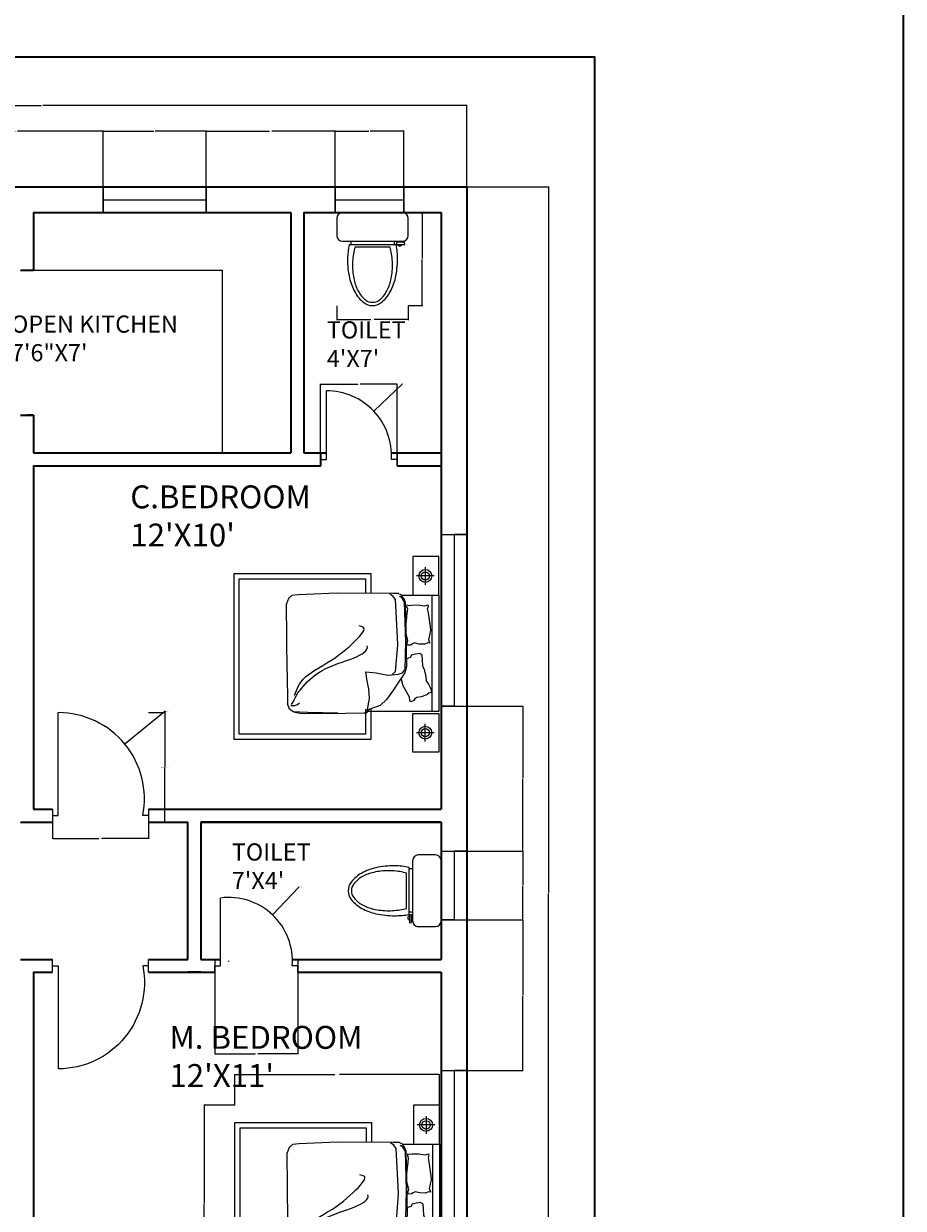
# Model space of a CAD drawing. Units: inches. Extents: x 1976 to 2558, y -977 to 2909.
# Tile 6 of 8: x 2251 to 2558, y 2026 to 2441. Entities that reach past the tile are written whole.
import ezdxf

# ---------------------------------------------------------------- set-up
doc = ezdxf.new("R2010")
doc.units = ezdxf.units.IN
for name, color, linetype, lineweight in [('A-ANNO-DIMS', 2, 'Continuous', 18), ('A-ANNO-TTLB', 7, 'Continuous', 35), ('A-AREA-IDEN', 7, 'Continuous', 18), ('A-DOOR', 3, 'Continuous', 18), ('A-FLOR-FIXT', 9, 'Continuous', 18), ('A-FURN', 8, 'Continuous', 13), ('A-GLAZ', 4, 'Continuous', 18), ('A-WALL', 7, 'Continuous', 35)]:
    doc.layers.add(name, color=color, linetype=linetype, lineweight=lineweight)
doc.styles.get("Standard").update_dxf_attribs({"font": 'arial.ttf'})
doc.dimstyles.get("Standard").update_dxf_attribs({"dimtxt": 0.18, "dimasz": 0.18, "dimexe": 0.18, "dimexo": 0.0625, "dimgap": 0.09, "dimtad": 0, "dimtih": 1, "dimtoh": 1, "dimdec": 4, "dimzin": 0, "dimdsep": 46, "dimtxsty": 'Standard', "dimcen": 0.09, "dimadec": 0, "dimazin": 0, "dimtfac": 1, "dimtdec": 4, "dimtofl": 0, "dimtmove": 0, "dimatfit": 3, "dimfxl": 1, "dimtolj": 1, "dimtzin": 0, "dimarcsym": 0})

# ---------------------------------------------------------------- blocks, each defined once
blk = doc.blocks.new('A$C238700B9')
for p, q in [((0, 0.61), (0, 0.49)), ((0.25, 0.65), (0.04, 0.65)), ((0.46, 0.65), (0.25, 0.65)), ((0.5, 0.49), (0.5, 0.61)), ((0.04, 0.45), (0.46, 0.45)), ((0.4166, 0.4252), (0.0876, 0.4252)), ((0.0974, 0.45), (0.0974, 0.4252)), ((0.401, 0.45), (0.401, 0.4252)), ((0.473, 0.4434), (0.419, 0.4434)), ((0.419, 0.4434), (0.419, 0.428)), ((0.419, 0.428), (0.4756, 0.428)), ((0.4337, 0.4434), (0.4337, 0.45)), ((0.446, 0.45), (0.446, 0.4434)), ((0.4756, 0.428), (0.473, 0.4434)), ((0.3733, 0.4074), (0.1267, 0.4074))]:
    blk.add_line(p, q)
for centre, radius, start, end in [((0.04, 0.61), 0.04, 90, 180), ((0.46, 0.61), 0.04, 0, 90), ((0.04, 0.49), 0.04, 180, 270), ((0.6767, 0.3001), 0.6022, 168.01944, 177.63471), ((-0.1767, 0.325), 0.6017, 0, 9.58156), ((0.4403, 0.434), 0.0169, 200.63996, 339.36004), ((0.46, 0.49), 0.04, 270, 0), ((0.5914, 0.2827), 0.4814, 167.42665, 180), ((0.4225, 0.3203), 0.3083, 163.59544, 167.42665), ((0.0775, 0.3203), 0.3083, 12.57335, 16.40456), ((-0.0914, 0.2827), 0.4814, 0, 12.57335), ((0.6767, 0.325), 0.6017, 180, 192.57335), ((0.5914, 0.2827), 0.4814, 180, 192.57335), ((-0.0914, 0.2827), 0.4814, 347.42665, 0), ((-0.1767, 0.325), 0.6017, 347.42665, 0), ((0.4656, 0.2779), 0.3854, 192.57335, 208.30076), ((0.4225, 0.245), 0.3083, 192.57335, 208.30076), ((0.0775, 0.245), 0.3083, 331.69924, 347.42665), ((0.0344, 0.2779), 0.3854, 331.69924, 347.42665), ((0.3327, 0.2064), 0.2345, 208.30076, 232.43058), ((0.3162, 0.1878), 0.1876, 208.30076, 232.43058), ((0.1838, 0.1878), 0.1876, 307.56942, 331.69924), ((0.1673, 0.2064), 0.2345, 307.56942, 331.69924), ((0.25, 0.0988), 0.0988, 232.43058, 270), ((0.2463, 0.0908), 0.0682, 229.31665, 273.11393), ((0.2537, 0.0908), 0.0682, 266.88607, 310.68335), ((0.25, 0.0988), 0.0988, 270, 307.56942)]:
    blk.add_arc(centre, radius, start, end)
blk = doc.blocks.new('BED-DOUBLE')
for p, q in [((66.8, 64.69), (66.8, 58.55)), ((69.87, 61.62), (63.73, 61.62)), ((20.15, 54.74), (18.94, 53.75)), ((22.42, 54.99), (20.15, 54.74)), ((25.18, 55.14), (22.42, 54.99)), ((35.73, 55.56), (25.18, 55.14)), ((55.41, 55.48), (35.73, 55.56)), ((56.88, 55.5), (55.41, 55.48)), ((57.51, 55.44), (56.88, 55.5)), ((58.41, 54.87), (71.47, 54.87)), ((18.94, 53.75), (18.3, 51.82)), ((18.55, 28.1), (18.3, 51.82)), ((66.5, 51.13), (67.81, 51.48)), ((60.75, 39.09), (59.91, 42.39)), ((68.04, 39.26), (68.74, 42.58)), ((68.74, 42.58), (68.6, 43.82)), ((60.42, 38.05), (60.75, 39.09)), ((60.63, 37.41), (60.42, 38.05)), ((61.72, 37.48), (60.63, 37.41)), ((62.3, 37.93), (61.72, 37.48)), ((63.04, 38.19), (62.3, 37.93)), ((64.58, 37.82), (63.04, 38.19)), ((66.65, 37.8), (64.58, 37.82)), ((67.64, 38.21), (66.65, 37.8)), ((68.39, 38.13), (67.64, 38.21)), ((68.39, 38.13), (67.64, 38.21)), ((68.42, 38.23), (68.04, 39.26)), ((68.39, 38.13), (68.42, 38.23)), ((65.64, 33.99), (65.86, 30.18)), ((65.86, 30.18), (66.35, 28.89)), ((18.55, 28.1), (18.55, 23.26)), ((66.35, 28.89), (67.01, 26.44)), ((67.01, 26.44), (67.13, 25.01)), ((67.13, 25.01), (67.97, 23.75)), ((67.13, 25.01), (67.97, 23.75)), ((18.55, 23.26), (18.68, 21.54)), ((18.68, 21.54), (18.68, 17.02)), ((61.33, 19.24), (59.08, 23.24)), ((68.1, 20.74), (67.32, 20.02)), ((67.97, 23.75), (68.81, 21.95)), ((19.39, 15.11), (18.68, 17.02)), ((21.2, 16.35), (22.12, 16.65)), ((22.12, 16.65), (22.82, 17.31)), ((61.37, 18.14), (61.33, 19.24)), ((61.78, 17.61), (61.37, 18.14)), ((62.78, 18.04), (61.78, 17.61)), ((63.18, 18.67), (62.78, 18.04)), ((63.79, 19.16), (63.18, 18.67)), ((65.36, 19.33), (63.79, 19.16)), ((67.32, 20.02), (65.36, 19.33)), ((20.62, 14.15), (19.39, 15.11)), ((19.85, 16.29), (21.2, 16.35)), ((22.9, 13.97), (20.62, 14.15)), ((21.04, 14.04), (23.05, 13.66)), ((25.67, 13.91), (22.9, 13.97)), ((23.05, 13.66), (24.99, 13.54)), ((24.99, 13.54), (38.97, 13.68)), ((36.23, 13.64), (25.67, 13.91)), ((38.97, 13.68), (45.35, 13.75)), ((46.53, 14.29), (46.57, 14.2)), ((66.8, 3.77), (66.8, 9.91)), ((69.87, 6.84), (63.73, 6.84))]:
    blk.add_line(p, q)
for points in [[(62.44, 68.46), (62.44, 54.92), (71.47, 54.92), (71.47, 68.46)], [(62.44, 0), (62.44, 13.54), (71.47, 13.54), (71.47, 0)]]:
    blk.add_lwpolyline(points, close=True)
for points in [[(47.73, 15.09), (47.73, 4.46), (0, 4.46), (0, 62.42), (47.73, 62.42), (47.73, 55.51)], [(45.92, 15.09), (45.92, 6.27), (1.81, 6.27), (1.81, 60.61), (45.92, 60.61), (45.92, 55.51)], [(46.51, 14.22), (47.31, 18.77), (47.06, 22.14), (46.5, 24.88), (46.05, 28.14), (49.6, 27.7), (53.74, 26.97), (57.39, 27.29), (58.87, 27.77), (59.72, 28.96), (59.98, 38.59), (59.57, 52.44), (58.73, 53.86), (57.9, 54.46), (57.82, 54.53)], [(58.65, 54.52), (59.13, 53.97), (59.77, 52.45), (60.21, 29.99), (59.63, 27.73), (57.24, 24.13), (55.74, 21.86), (53.24, 18.45), (51.03, 16.28), (47.47, 15), (46.54, 14.37)], [(71.47, 54.87), (71.47, 14.22), (46.61, 14.22)], [(55.37, 27.24), (56.41, 28.26), (57.19, 37.43), (57.04, 40.1), (56.37, 53.37), (55.53, 54.49), (54.4, 55.34)], [(57.55, 55.42), (57.97, 55.29), (58.3, 55.1), (58.41, 54.87), (58.64, 54.6), (58.65, 54.56)], [(69.21, 14.22), (69.21, 54.87)], [(59.99, 43.62), (60.51, 48.57), (60.69, 50), (60.38, 50.84), (60.47, 51.53), (61.01, 51.34), (61.95, 51.45), (64.12, 51.49), (66.5, 51.18)], [(68.6, 43.82), (67.86, 48.73), (67.62, 50.16), (67.9, 51.01), (67.81, 51.48)], [(21.07, 19.9), (21.44, 20.76), (21.79, 21.6), (22.14, 22.42), (22.52, 23.22), (22.95, 24.01), (23.48, 24.78), (24.13, 25.56), (24.93, 26.33), (25.9, 27.1), (27.01, 27.89), (28.25, 28.69), (29.59, 29.5), (30.98, 30.34), (32.41, 31.2), (33.84, 32.1), (35.25, 33.03), (36.61, 34), (37.91, 35), (39.14, 36), (40.28, 37), (41.34, 37.97), (42.3, 38.91), (43.16, 39.79), (43.9, 40.61), (44.52, 41.34), (44.99, 41.98), (45.3, 42.54), (45.43, 43.02), (45.35, 43.42), (45.05, 43.74), (44.51, 43.98), (43.7, 44.14)], [(20, 16.69), (20.29, 17.07), (20.52, 17.41), (20.72, 17.72), (20.88, 18.01), (21.02, 18.28), (21.14, 18.55), (21.26, 18.81), (21.37, 19.07), (21.5, 19.34), (21.64, 19.63), (21.82, 19.96), (22.04, 20.32), (22.31, 20.72), (22.64, 21.19), (23.05, 21.72), (23.54, 22.32), (24.12, 23.01), (24.8, 23.76), (25.57, 24.56), (26.43, 25.38), (27.39, 26.22), (28.43, 27.04), (29.56, 27.83), (30.78, 28.58), (32.09, 29.26), (33.45, 29.88), (34.86, 30.45), (36.28, 30.99), (37.7, 31.49), (39.08, 31.98), (40.41, 32.45), (41.66, 32.92), (42.81, 33.4), (43.84, 33.89), (44.73, 34.4), (45.46, 34.92), (46.02, 35.46), (46.39, 36.02), (46.55, 36.61), (46.48, 37.23)], [(65.64, 33.99), (64.89, 34.52), (63.32, 34.27), (61.94, 33.89), (61.5, 33.14), (60.37, 32.7), (60.16, 32.7)], [(59.08, 23.24), (58.42, 25.91)], [(68.1, 20.74), (68.93, 20.99), (69.11, 21.53), (68.81, 21.95)], [(45.41, 13.75), (46.29, 13.81), (46.55, 14.07), (46.61, 14.22)]]:
    blk.add_lwpolyline(points)
for centre, radius in [((66.8, 61.62), 2.26), ((66.8, 61.62), 1.45), ((66.8, 6.84), 2.26), ((66.8, 6.84), 1.45)]:
    blk.add_circle(centre, radius)
blk = doc.blocks.new('DOOR-BEDROOM')
for p, q in [((2, 2.25), (2, 38.25)), ((0, 4.5), (0, 0)), ((33.52, 4.5), (33.52, 0)), ((0, 2.25), (2, 2.25)), ((33.52, 2.25), (31.52, 2.25))]:
    blk.add_line(p, q)
blk.add_arc((2, 8.15), 30.1, 348.694, 90)
blk = doc.blocks.new('WIN-60-PLAN')
for p, q in [((4.5, 60), (0, 60)), ((0, 60), (9, 60)), ((4.5, 0), (4.5, 60)), ((0, 0), (9, 0)), ((9, 0), (4.5, 0))]:
    blk.add_line(p, q)
blk = doc.blocks.new('*D13')
at = {"layer": 'A-ANNO-DIMS', "color": 0, "lineweight": -2, "transparency": 16777216}
for p, q in [((2384.99, 2374.48), (2389.98, 2374.48)), ((2389.8, 2374.3), (2389.8, 2358.43)), ((2389.8, 2342.19), (2389.8, 2358.06)), ((2384.99, 2342.01), (2389.98, 2342.01))]:
    blk.add_line(p, q, dxfattribs=at)
at = {"layer": 'A-ANNO-DIMS', "color": 0, "transparency": 16777216}
for points in [[(2389.77, 2374.3), (2389.83, 2374.3), (2389.8, 2374.48)], [(2389.77, 2342.19), (2389.83, 2342.19), (2389.8, 2342.01)]]:
    blk.add_solid(points, dxfattribs=at)
at = {"layer": 'Defpoints', "color": 0, "transparency": 16777216}
for p in [(2384.93, 2374.48), (2389.8, 2374.48), (2384.93, 2342.01)]:
    blk.add_point(p, dxfattribs=at)
at = {"layer": 'A-ANNO-DIMS', "color": 0, "transparency": 16777216, "insert": (2389.8, 2358.24), "char_height": 0.18, "attachment_point": 5}
blk.add_mtext('\\A1;WC 32 TYP.', dxfattribs=at)
blk = doc.blocks.new('*D14')
at = {"layer": 'A-ANNO-DIMS', "color": 0, "lineweight": -2, "transparency": 16777216}
for p, q in [((2359.95, 2341.94), (2359.95, 2336.95)), ((2384.93, 2341.94), (2384.93, 2336.95)), ((2360.13, 2337.13), (2371.91, 2337.13)), ((2384.75, 2337.13), (2372.97, 2337.13))]:
    blk.add_line(p, q, dxfattribs=at)
at = {"layer": 'A-ANNO-DIMS', "color": 0, "transparency": 16777216}
for points in [[(2360.13, 2337.16), (2360.13, 2337.1), (2359.95, 2337.13)], [(2384.75, 2337.16), (2384.75, 2337.1), (2384.93, 2337.13)]]:
    blk.add_solid(points, dxfattribs=at)
at = {"layer": 'Defpoints', "color": 0, "transparency": 16777216}
for p in [(2359.95, 2342.01), (2384.93, 2342.01), (2384.93, 2337.13)]:
    blk.add_point(p, dxfattribs=at)
at = {"layer": 'A-ANNO-DIMS', "color": 0, "transparency": 16777216, "insert": (2372.44, 2337.13), "char_height": 0.18, "attachment_point": 5}
blk.add_mtext('\\A1;25 TYP.', dxfattribs=at)
blk = doc.blocks.new('*D15')
at = {"layer": 'A-ANNO-DIMS', "color": 0, "lineweight": -2, "transparency": 16777216}
for p, q in [((2324.36, 2062.54), (2324.36, 2073.38)), ((2324.54, 2073.2), (2359.28, 2073.2)), ((2395.66, 2073.2), (2360.92, 2073.2)), ((2395.84, 2062.54), (2395.84, 2073.38))]:
    blk.add_line(p, q, dxfattribs=at)
at = {"layer": 'A-ANNO-DIMS', "color": 0, "transparency": 16777216}
for points in [[(2324.54, 2073.23), (2324.54, 2073.17), (2324.36, 2073.2)], [(2395.66, 2073.23), (2395.66, 2073.17), (2395.84, 2073.2)]]:
    blk.add_solid(points, dxfattribs=at)
at = {"layer": 'Defpoints', "color": 0, "transparency": 16777216}
for p in [(2395.84, 2073.2), (2324.36, 2062.48), (2395.84, 2062.48)]:
    blk.add_point(p, dxfattribs=at)
at = {"layer": 'A-ANNO-DIMS', "color": 0, "transparency": 16777216, "insert": (2360.1, 2073.2), "char_height": 0.18, "attachment_point": 5}
blk.add_mtext('\\A1;BED 71 TYP.', dxfattribs=at)
blk = doc.blocks.new('*D16')
at = {"layer": 'A-ANNO-DIMS', "color": 0, "lineweight": -2, "transparency": 16777216}
for p, q in [((2324.3, 2062.48), (2313.46, 2062.48)), ((2313.64, 2062.3), (2313.64, 2028.43)), ((2313.64, 1994.19), (2313.64, 2028.06)), ((2324.3, 1994.01), (2313.46, 1994.01))]:
    blk.add_line(p, q, dxfattribs=at)
at = {"layer": 'A-ANNO-DIMS', "color": 0, "transparency": 16777216}
for points in [[(2313.61, 2062.3), (2313.67, 2062.3), (2313.64, 2062.48)], [(2313.61, 1994.19), (2313.67, 1994.19), (2313.64, 1994.01)]]:
    blk.add_solid(points, dxfattribs=at)
at = {"layer": 'Defpoints', "color": 0, "transparency": 16777216}
for p in [(2313.64, 2062.48), (2324.36, 2062.48), (2324.36, 1994.01)]:
    blk.add_point(p, dxfattribs=at)
at = {"layer": 'A-ANNO-DIMS', "color": 0, "transparency": 16777216, "insert": (2313.64, 2028.25), "char_height": 0.18, "attachment_point": 5}
blk.add_mtext('\\A1;68 TYP.', dxfattribs=at)
blk = doc.blocks.new('*D19')
at = {"layer": 'A-ANNO-DIMS', "color": 0, "lineweight": -2, "transparency": 16777216}
for p, q in [((2294.21, 2199.73), (2300.07, 2199.73)), ((2299.89, 2199.55), (2299.89, 2180.79)), ((2299.89, 2161.66), (2299.89, 2180.42)), ((2294.21, 2161.48), (2300.07, 2161.48))]:
    blk.add_line(p, q, dxfattribs=at)
at = {"layer": 'A-ANNO-DIMS', "color": 0, "transparency": 16777216}
for points in [[(2299.86, 2199.55), (2299.92, 2199.55), (2299.89, 2199.73)], [(2299.86, 2161.66), (2299.92, 2161.66), (2299.89, 2161.48)]]:
    blk.add_solid(points, dxfattribs=at)
at = {"layer": 'Defpoints', "color": 0, "transparency": 16777216}
for p in [(2294.15, 2199.73), (2299.89, 2199.73), (2294.15, 2161.48)]:
    blk.add_point(p, dxfattribs=at)
at = {"layer": 'A-ANNO-DIMS', "color": 0, "transparency": 16777216, "insert": (2299.89, 2180.6), "char_height": 0.18, "attachment_point": 5}
blk.add_mtext('\\A1;BEDROOM DOOR 38 TYP.', dxfattribs=at)
blk = doc.blocks.new('*D20')
at = {"layer": 'A-ANNO-DIMS', "color": 0, "lineweight": -2, "transparency": 16777216}
for p, q in [((2260.63, 2161.42), (2260.63, 2155.56)), ((2294.15, 2161.42), (2294.15, 2155.56)), ((2260.81, 2155.74), (2276.86, 2155.74)), ((2293.97, 2155.74), (2277.92, 2155.74))]:
    blk.add_line(p, q, dxfattribs=at)
at = {"layer": 'A-ANNO-DIMS', "color": 0, "transparency": 16777216}
for points in [[(2260.81, 2155.77), (2260.81, 2155.71), (2260.63, 2155.74)], [(2293.97, 2155.77), (2293.97, 2155.71), (2294.15, 2155.74)]]:
    blk.add_solid(points, dxfattribs=at)
at = {"layer": 'Defpoints', "color": 0, "transparency": 16777216}
for p in [(2260.63, 2161.48), (2294.15, 2161.48), (2294.15, 2155.74)]:
    blk.add_point(p, dxfattribs=at)
at = {"layer": 'A-ANNO-DIMS', "color": 0, "transparency": 16777216, "insert": (2277.39, 2155.74), "char_height": 0.18, "attachment_point": 5}
blk.add_mtext('\\A1;34 TYP.', dxfattribs=at)
blk = doc.blocks.new('*D23')
at = {"layer": 'A-ANNO-DIMS', "color": 0, "lineweight": -2, "transparency": 16777216}
for p, q in [((2108.44, 2383.54), (2108.44, 2412.16)), ((2108.62, 2411.98), (2256.65, 2411.98)), ((2405.26, 2411.98), (2257.23, 2411.98)), ((2405.44, 2383.54), (2405.44, 2412.16))]:
    blk.add_line(p, q, dxfattribs=at)
at = {"layer": 'A-ANNO-DIMS', "color": 0, "transparency": 16777216}
for points in [[(2108.62, 2412.01), (2108.62, 2411.95), (2108.44, 2411.98)], [(2405.26, 2412.01), (2405.26, 2411.95), (2405.44, 2411.98)]]:
    blk.add_solid(points, dxfattribs=at)
at = {"layer": 'Defpoints', "color": 0, "transparency": 16777216}
for p in [(2405.44, 2411.98), (2108.44, 2383.48), (2405.44, 2383.48)]:
    blk.add_point(p, dxfattribs=at)
at = {"layer": 'A-ANNO-DIMS', "color": 0, "transparency": 16777216, "insert": (2256.94, 2411.98), "char_height": 0.18, "attachment_point": 5}
blk.add_mtext('\\A1;297', dxfattribs=at)
blk = doc.blocks.new('*D24')
at = {"layer": 'A-ANNO-DIMS', "color": 0, "lineweight": -2, "transparency": 16777216}
for p, q in [((2405.5, 2383.48), (2434.12, 2383.48)), ((2433.94, 2383.3), (2433.94, 2136.91)), ((2433.94, 1890.16), (2433.94, 2136.55)), ((2359.5, 1889.98), (2434.12, 1889.98))]:
    blk.add_line(p, q, dxfattribs=at)
at = {"layer": 'A-ANNO-DIMS', "color": 0, "transparency": 16777216}
for points in [[(2433.91, 2383.3), (2433.97, 2383.3), (2433.94, 2383.48)], [(2433.91, 1890.16), (2433.97, 1890.16), (2433.94, 1889.98)]]:
    blk.add_solid(points, dxfattribs=at)
at = {"layer": 'Defpoints', "color": 0, "transparency": 16777216}
for p in [(2405.44, 2383.48), (2433.94, 2383.48), (2359.44, 1889.98)]:
    blk.add_point(p, dxfattribs=at)
at = {"layer": 'A-ANNO-DIMS', "color": 0, "transparency": 16777216, "insert": (2433.94, 2136.73), "char_height": 0.18, "attachment_point": 5}
blk.add_mtext('\\A1;493.5', dxfattribs=at)
blk = doc.blocks.new('*D29')
at = {"layer": 'A-ANNO-DIMS', "color": 0, "lineweight": -2, "transparency": 16777216}
for p, q in [((2217.76, 2374.54), (2217.76, 2403.16)), ((2217.94, 2402.98), (2247.63, 2402.98)), ((2278.11, 2402.98), (2248.42, 2402.98)), ((2278.29, 2374.54), (2278.29, 2403.16))]:
    blk.add_line(p, q, dxfattribs=at)
at = {"layer": 'A-ANNO-DIMS', "color": 0, "transparency": 16777216}
for points in [[(2217.94, 2403.01), (2217.94, 2402.95), (2217.76, 2402.98)], [(2278.11, 2403.01), (2278.11, 2402.95), (2278.29, 2402.98)]]:
    blk.add_solid(points, dxfattribs=at)
at = {"layer": 'Defpoints', "color": 0, "transparency": 16777216}
for p in [(2278.29, 2402.98), (2217.76, 2374.48), (2278.29, 2374.48)]:
    blk.add_point(p, dxfattribs=at)
at = {"layer": 'A-ANNO-DIMS', "color": 0, "transparency": 16777216, "insert": (2248.02, 2402.98), "char_height": 0.18, "attachment_point": 5}
blk.add_mtext('\\A1;60.53', dxfattribs=at)
blk = doc.blocks.new('*D30')
at = {"layer": 'A-ANNO-DIMS', "color": 0, "lineweight": -2, "transparency": 16777216}
for p, q in [((2278.29, 2374.54), (2278.29, 2403.16)), ((2278.47, 2402.98), (2296.07, 2402.98)), ((2314.11, 2402.98), (2296.51, 2402.98)), ((2314.29, 2374.54), (2314.29, 2403.16))]:
    blk.add_line(p, q, dxfattribs=at)
at = {"layer": 'A-ANNO-DIMS', "color": 0, "transparency": 16777216}
for points in [[(2278.47, 2403.01), (2278.47, 2402.95), (2278.29, 2402.98)], [(2314.11, 2403.01), (2314.11, 2402.95), (2314.29, 2402.98)]]:
    blk.add_solid(points, dxfattribs=at)
at = {"layer": 'Defpoints', "color": 0, "transparency": 16777216}
for p in [(2314.29, 2402.98), (2278.29, 2374.48), (2314.29, 2374.48)]:
    blk.add_point(p, dxfattribs=at)
at = {"layer": 'A-ANNO-DIMS', "color": 0, "transparency": 16777216, "insert": (2296.29, 2402.98), "char_height": 0.18, "attachment_point": 5}
blk.add_mtext('\\A1;36', dxfattribs=at)
blk = doc.blocks.new('*D31')
at = {"layer": 'A-ANNO-DIMS', "color": 0, "lineweight": -2, "transparency": 16777216}
for p, q in [((2314.29, 2374.54), (2314.29, 2403.16)), ((2314.47, 2402.98), (2336.46, 2402.98)), ((2359.21, 2402.98), (2337.22, 2402.98)), ((2359.39, 2374.54), (2359.39, 2403.16))]:
    blk.add_line(p, q, dxfattribs=at)
at = {"layer": 'A-ANNO-DIMS', "color": 0, "transparency": 16777216}
for points in [[(2314.47, 2403.01), (2314.47, 2402.95), (2314.29, 2402.98)], [(2359.21, 2403.01), (2359.21, 2402.95), (2359.39, 2402.98)]]:
    blk.add_solid(points, dxfattribs=at)
at = {"layer": 'Defpoints', "color": 0, "transparency": 16777216}
for p in [(2359.39, 2402.98), (2314.29, 2374.48), (2359.39, 2374.48)]:
    blk.add_point(p, dxfattribs=at)
at = {"layer": 'A-ANNO-DIMS', "color": 0, "transparency": 16777216, "insert": (2336.84, 2402.98), "char_height": 0.18, "attachment_point": 5}
blk.add_mtext('\\A1;45.11', dxfattribs=at)
blk = doc.blocks.new('*D32')
at = {"layer": 'A-ANNO-DIMS', "color": 0, "lineweight": -2, "transparency": 16777216}
for p, q in [((2359.39, 2374.54), (2359.39, 2403.16)), ((2359.57, 2402.98), (2371.17, 2402.98)), ((2383.21, 2402.98), (2371.61, 2402.98)), ((2383.39, 2374.54), (2383.39, 2403.16))]:
    blk.add_line(p, q, dxfattribs=at)
at = {"layer": 'A-ANNO-DIMS', "color": 0, "transparency": 16777216}
for points in [[(2359.57, 2403.01), (2359.57, 2402.95), (2359.39, 2402.98)], [(2383.21, 2403.01), (2383.21, 2402.95), (2383.39, 2402.98)]]:
    blk.add_solid(points, dxfattribs=at)
at = {"layer": 'Defpoints', "color": 0, "transparency": 16777216}
for p in [(2383.39, 2402.98), (2359.39, 2374.48), (2383.39, 2374.48)]:
    blk.add_point(p, dxfattribs=at)
at = {"layer": 'A-ANNO-DIMS', "color": 0, "transparency": 16777216, "insert": (2371.39, 2402.98), "char_height": 0.18, "attachment_point": 5}
blk.add_mtext('\\A1;24', dxfattribs=at)
blk = doc.blocks.new('*D38')
at = {"layer": 'A-ANNO-DIMS', "color": 0, "lineweight": -2, "transparency": 16777216}
for p, q in [((2396.5, 2127.29), (2425.12, 2127.29)), ((2424.94, 2127.11), (2424.94, 2101.14)), ((2424.94, 2074.8), (2424.94, 2100.77)), ((2396.5, 2074.62), (2425.12, 2074.62))]:
    blk.add_line(p, q, dxfattribs=at)
at = {"layer": 'A-ANNO-DIMS', "color": 0, "transparency": 16777216}
for points in [[(2424.91, 2127.11), (2424.97, 2127.11), (2424.94, 2127.29)], [(2424.91, 2074.8), (2424.97, 2074.8), (2424.94, 2074.62)]]:
    blk.add_solid(points, dxfattribs=at)
at = {"layer": 'Defpoints', "color": 0, "transparency": 16777216}
for p in [(2396.44, 2127.29), (2396.44, 2074.62), (2424.94, 2074.62)]:
    blk.add_point(p, dxfattribs=at)
at = {"layer": 'A-ANNO-DIMS', "color": 0, "transparency": 16777216, "insert": (2424.94, 2100.95), "char_height": 0.18, "attachment_point": 5}
blk.add_mtext('\\A1;52.67', dxfattribs=at)
blk = doc.blocks.new('*D39')
at = {"layer": 'A-ANNO-DIMS', "color": 0, "lineweight": -2, "transparency": 16777216}
for p, q in [((2396.5, 2151.29), (2425.12, 2151.29)), ((2424.94, 2151.11), (2424.94, 2139.47)), ((2424.94, 2127.47), (2424.94, 2139.11)), ((2396.5, 2127.29), (2425.12, 2127.29))]:
    blk.add_line(p, q, dxfattribs=at)
at = {"layer": 'A-ANNO-DIMS', "color": 0, "transparency": 16777216}
for points in [[(2424.91, 2151.11), (2424.97, 2151.11), (2424.94, 2151.29)], [(2424.91, 2127.47), (2424.97, 2127.47), (2424.94, 2127.29)]]:
    blk.add_solid(points, dxfattribs=at)
at = {"layer": 'Defpoints', "color": 0, "transparency": 16777216}
for p in [(2396.44, 2151.29), (2396.44, 2127.29), (2424.94, 2127.29)]:
    blk.add_point(p, dxfattribs=at)
at = {"layer": 'A-ANNO-DIMS', "color": 0, "transparency": 16777216, "insert": (2424.94, 2139.29), "char_height": 0.18, "attachment_point": 5}
blk.add_mtext('\\A1;24', dxfattribs=at)
blk = doc.blocks.new('*D40')
at = {"layer": 'A-ANNO-DIMS', "color": 0, "lineweight": -2, "transparency": 16777216}
for p, q in [((2396.5, 2201.99), (2425.12, 2201.99)), ((2424.94, 2201.81), (2424.94, 2176.82)), ((2424.94, 2151.47), (2424.94, 2176.46)), ((2396.5, 2151.29), (2425.12, 2151.29))]:
    blk.add_line(p, q, dxfattribs=at)
at = {"layer": 'A-ANNO-DIMS', "color": 0, "transparency": 16777216}
for points in [[(2424.91, 2201.81), (2424.97, 2201.81), (2424.94, 2201.99)], [(2424.91, 2151.47), (2424.97, 2151.47), (2424.94, 2151.29)]]:
    blk.add_solid(points, dxfattribs=at)
at = {"layer": 'Defpoints', "color": 0, "transparency": 16777216}
for p in [(2396.44, 2201.99), (2396.44, 2151.29), (2424.94, 2151.29)]:
    blk.add_point(p, dxfattribs=at)
at = {"layer": 'A-ANNO-DIMS', "color": 0, "transparency": 16777216, "insert": (2424.94, 2176.64), "char_height": 0.18, "attachment_point": 5}
blk.add_mtext('\\A1;50.7', dxfattribs=at)
blk = doc.blocks.new('*D47')
at = {"layer": 'A-ANNO-DIMS', "color": 0, "lineweight": -2, "transparency": 16777216}
for p, q in [((2354.33, 2286.04), (2354.33, 2314.66)), ((2381.08, 2286.04), (2381.08, 2314.66)), ((2354.51, 2314.48), (2367.31, 2314.48)), ((2380.9, 2314.48), (2368.1, 2314.48))]:
    blk.add_line(p, q, dxfattribs=at)
at = {"layer": 'A-ANNO-DIMS', "color": 0, "transparency": 16777216}
for points in [[(2354.51, 2314.51), (2354.51, 2314.45), (2354.33, 2314.48)], [(2380.9, 2314.51), (2380.9, 2314.45), (2381.08, 2314.48)]]:
    blk.add_solid(points, dxfattribs=at)
at = {"layer": 'Defpoints', "color": 0, "transparency": 16777216}
for p in [(2381.08, 2314.48), (2354.33, 2285.98), (2381.08, 2285.98)]:
    blk.add_point(p, dxfattribs=at)
at = {"layer": 'A-ANNO-DIMS', "color": 0, "transparency": 16777216, "insert": (2367.71, 2314.48), "char_height": 0.18, "attachment_point": 5}
blk.add_mtext('\\A1;26.75', dxfattribs=at)
blk = doc.blocks.new('*D48')
at = {"layer": 'A-ANNO-DIMS', "color": 0, "lineweight": -2, "transparency": 16777216}
for p, q in [((2317.31, 2108.92), (2317.31, 2080.3)), ((2346.41, 2108.92), (2346.41, 2080.3)), ((2317.49, 2080.48), (2331.4, 2080.48)), ((2346.23, 2080.48), (2332.33, 2080.48))]:
    blk.add_line(p, q, dxfattribs=at)
at = {"layer": 'A-ANNO-DIMS', "color": 0, "transparency": 16777216}
for points in [[(2317.49, 2080.51), (2317.49, 2080.45), (2317.31, 2080.48)], [(2346.23, 2080.51), (2346.23, 2080.45), (2346.41, 2080.48)]]:
    blk.add_solid(points, dxfattribs=at)
at = {"layer": 'Defpoints', "color": 0, "transparency": 16777216}
for p in [(2317.31, 2108.98), (2346.41, 2108.98), (2317.31, 2080.48)]:
    blk.add_point(p, dxfattribs=at)
at = {"layer": 'A-ANNO-DIMS', "color": 0, "transparency": 16777216, "insert": (2331.86, 2080.48), "char_height": 0.18, "attachment_point": 5}
blk.add_mtext('\\A1;29.097', dxfattribs=at)
blk = doc.blocks.new('*D90')
at = {"layer": 'A-ANNO-DIMS', "color": 0, "lineweight": -2, "transparency": 16777216}
for p, q in [((2299.88, 2200.16), (2286.05, 2188.83)), ((2300.06, 2200.16), (2299.88, 2200.16)), ((2262.54, 2169.63), (2262.72, 2169.63)), ((2262.63, 2169.54), (2262.63, 2169.72))]:
    blk.add_line(p, q, dxfattribs=at)
at = {"layer": 'A-ANNO-DIMS', "color": 0, "transparency": 16777216}
blk.add_solid([(2286.03, 2188.85), (2286.07, 2188.8), (2285.91, 2188.71)], dxfattribs=at)
at = {"layer": 'Defpoints', "color": 0, "transparency": 16777216}
for p in [(2285.91, 2188.71), (2262.63, 2169.63)]:
    blk.add_point(p, dxfattribs=at)
at = {"layer": 'A-ANNO-DIMS', "color": 0, "transparency": 16777216, "insert": (2300.64, 2200.16), "char_height": 0.18, "attachment_point": 5}
blk.add_mtext('\\A1;2X R30.1', dxfattribs=at)
blk = doc.blocks.new('*D91')
at = {"layer": 'A-ANNO-DIMS', "color": 0, "lineweight": -2, "transparency": 16777216}
for p, q in [((2382.79, 2314.52), (2373, 2305.24)), ((2382.97, 2314.52), (2382.79, 2314.52)), ((2356.24, 2289.45), (2356.42, 2289.45)), ((2356.33, 2289.36), (2356.33, 2289.54))]:
    blk.add_line(p, q, dxfattribs=at)
at = {"layer": 'A-ANNO-DIMS', "color": 0, "transparency": 16777216}
blk.add_solid([(2372.98, 2305.27), (2373.02, 2305.22), (2372.87, 2305.12)], dxfattribs=at)
at = {"layer": 'Defpoints', "color": 0, "transparency": 16777216}
for p in [(2372.87, 2305.12), (2356.33, 2289.45)]:
    blk.add_point(p, dxfattribs=at)
at = {"layer": 'A-ANNO-DIMS', "color": 0, "transparency": 16777216, "insert": (2383.45, 2314.52), "char_height": 0.18, "attachment_point": 5}
blk.add_mtext('\\A1;R22.78', dxfattribs=at)
blk = doc.blocks.new('*D92')
at = {"layer": 'A-ANNO-DIMS', "color": 0, "lineweight": -2, "transparency": 16777216}
for p, q in [((2346.66, 2138.75), (2337.63, 2129.19)), ((2346.84, 2138.75), (2346.66, 2138.75)), ((2322.16, 2112.9), (2322.34, 2112.9)), ((2322.25, 2112.81), (2322.25, 2112.99))]:
    blk.add_line(p, q, dxfattribs=at)
at = {"layer": 'A-ANNO-DIMS', "color": 0, "transparency": 16777216}
blk.add_solid([(2337.61, 2129.21), (2337.65, 2129.17), (2337.51, 2129.06)], dxfattribs=at)
at = {"layer": 'Defpoints', "color": 0, "transparency": 16777216}
for p in [(2337.51, 2129.06), (2322.25, 2112.9)]:
    blk.add_point(p, dxfattribs=at)
at = {"layer": 'A-ANNO-DIMS', "color": 0, "transparency": 16777216, "insert": (2347.32, 2138.75), "char_height": 0.18, "attachment_point": 5}
blk.add_mtext('\\A1;R22.22', dxfattribs=at)

msp = doc.modelspace()

# ---------------------------------------------------------------- linework, layer by layer
at = {"layer": 'A-ANNO-TTLB'}
for points in [[(1975.8545, 2909.3429), (2557.9168, 2909.3429), (2557.9168, 1747.8598), (1975.8545, 1747.8598)], [(2055.4343, 2428.9091), (2450.0007, 2428.9091), (2450.0007, 1815.3916), (2055.4343, 1815.3916)]]:
    msp.add_lwpolyline(points, close=True, dxfattribs=at)
at = {"layer": 'A-DOOR'}
for p, q in [((2356.3321, 2288.2289), (2356.3321, 2312.2289)), ((2354.3321, 2290.4789), (2354.3321, 2285.9789)), ((2381.0798, 2290.4789), (2381.0798, 2285.9789)), ((2354.3321, 2285.9789), (2354.3321, 2288.2289)), ((2354.3321, 2288.2289), (2356.3321, 2288.2289)), ((2381.0798, 2288.2289), (2379.0798, 2288.2289)), ((2381.0798, 2285.9789), (2381.0798, 2288.2289)), ((2319.3134, 2111.2289), (2319.3134, 2134.9248)), ((2317.3134, 2113.4789), (2317.3134, 2108.9789)), ((2346.4103, 2113.4789), (2346.4103, 2108.9789)), ((2294.1493, 2111.2289), (2294.1493, 2111.2289)), ((2317.3134, 2108.9789), (2317.3134, 2111.2289)), ((2317.3134, 2111.2289), (2319.3134, 2111.2289)), ((2346.4103, 2111.2289), (2344.4103, 2111.2289)), ((2346.4103, 2108.9789), (2346.4103, 2111.2289))]:
    msp.add_line(p, q, dxfattribs=at)
for centre, radius, start, end in [((2356.3321, 2289.4486), 22.7803, 356.930824, 90), ((2322.2509, 2112.8976), 22.2221, 355.693401, 97.596054)]:
    msp.add_arc(centre, radius, start, end, dxfattribs=at)
at = {"layer": 'A-FLOR-FIXT'}
for p, q in [((2253.9385, 2354.4047), (2319.9706, 2354.4047)), ((2319.9706, 2354.4047), (2319.9706, 2290.4789))]:
    msp.add_line(p, q, dxfattribs=at)
at = {"layer": 'A-GLAZ'}
for p, q in [((2278.2865, 2383.4789), (2278.2865, 2374.4789)), ((2314.2865, 2378.9789), (2314.2865, 2383.4789)), ((2314.2865, 2383.4789), (2314.2865, 2374.4789)), ((2359.3938, 2383.4789), (2359.3938, 2374.4789)), ((2383.3938, 2378.9789), (2383.3938, 2383.4789)), ((2383.3938, 2383.4789), (2383.3938, 2374.4789)), ((2278.2865, 2374.4789), (2278.2865, 2378.9789)), ((2278.2865, 2378.9789), (2314.2865, 2378.9789)), ((2359.3938, 2374.4789), (2359.3938, 2380.3577)), ((2359.3938, 2380.3577), (2359.3938, 2378.9789)), ((2359.3938, 2378.9789), (2383.3938, 2378.9789)), ((2396.4385, 2151.2893), (2405.4385, 2151.2893)), ((2405.4385, 2151.2893), (2400.9385, 2151.2893)), ((2400.9385, 2151.2893), (2400.9385, 2127.2893)), ((2400.9385, 2127.2893), (2396.4385, 2127.2893)), ((2396.4385, 2127.2893), (2405.4385, 2127.2893))]:
    msp.add_line(p, q, dxfattribs=at)
at = {"layer": 'A-WALL'}
for p, q in [((2108.4385, 2383.4789), (2405.4385, 2383.4789)), ((2405.4385, 2383.4789), (2405.4385, 1967.9789)), ((2253.9385, 2374.4789), (2253.9385, 2354.4047)), ((2253.9385, 2374.4789), (2343.9385, 2374.4789)), ((2343.9385, 2374.4789), (2343.9385, 2290.4789)), ((2348.4385, 2374.4789), (2348.4385, 2290.4789)), ((2348.4385, 2374.4789), (2396.4385, 2374.4789)), ((2396.4385, 2374.4789), (2396.4385, 2165.9789)), ((2249.4385, 2354.4047), (2253.9385, 2354.4047)), ((2249.4385, 2303.735), (2253.9385, 2303.735)), ((2253.9385, 2303.735), (2251.6885, 2303.735)), ((2251.6885, 2303.735), (2252.8135, 2303.735)), ((2253.9385, 2303.735), (2253.9385, 2290.4789)), ((2253.9385, 2290.4789), (2343.9385, 2290.4789)), ((2348.4385, 2290.4789), (2356.3321, 2290.4789)), ((2379.0891, 2290.4789), (2396.4385, 2290.4789)), ((2253.9385, 2285.9789), (2354.3321, 2285.9789)), ((2253.9385, 2285.9789), (2253.9385, 2165.9789)), ((2381.0798, 2285.9789), (2396.4385, 2285.9789)), ((2253.9385, 2165.9789), (2260.6343, 2165.9789)), ((2294.1493, 2165.9789), (2396.4385, 2165.9789)), ((2249.4385, 2161.4789), (2260.6343, 2161.4789)), ((2294.1493, 2161.4789), (2307.9385, 2161.4789)), ((2307.9385, 2113.4789), (2307.9385, 2161.4789)), ((2396.4385, 2161.4789), (2312.4385, 2161.4789)), ((2312.4385, 2161.4789), (2312.4385, 2113.4789)), ((2312.4385, 2161.4789), (2396.4385, 2161.4789)), ((2396.4385, 2161.4789), (2396.4385, 2113.4789)), ((2249.4385, 2113.4789), (2260.6343, 2113.4789)), ((2294.1493, 2113.4789), (2307.9385, 2113.4789)), ((2312.4385, 2113.4789), (2319.3134, 2113.4789)), ((2344.4655, 2113.4789), (2396.4385, 2113.4789)), ((2253.9385, 2108.9789), (2260.6343, 2108.9789)), ((2253.9385, 2108.9789), (2253.9385, 1976.9789)), ((2294.1493, 2108.9789), (2317.3134, 2108.9789)), ((2312.4385, 2108.9789), (2307.9385, 2108.9789)), ((2346.4103, 2108.9789), (2396.4385, 2108.9789)), ((2396.4385, 2108.9789), (2396.4385, 1976.9789))]:
    msp.add_line(p, q, dxfattribs=at)

# ---------------------------------------------------------------- block references
at = {"layer": 'A-DOOR'}
msp.add_blockref('DOOR-BEDROOM', (2260.634, 2161.479), dxfattribs=at)
at = {"layer": 'A-DOOR', "extrusion": (0, 0, -1), "zscale": -1, "rotation": 180}
msp.add_blockref('DOOR-BEDROOM', (-2260.634, 2113.4788), dxfattribs=at)
at = {"layer": 'A-FLOR-FIXT', "xscale": 49.9590227079487, "yscale": 49.9590227079487, "zscale": 49.9590227079487}
msp.add_blockref('A$C238700B9', (2359.9487, 2342.0055), dxfattribs=at)
at = {"layer": 'A-FLOR-FIXT', "xscale": 49.9590227079487, "yscale": 49.9590227079487, "zscale": 49.9590227079487, "rotation": 270}
msp.add_blockref('A$C238700B9', (2363.9651, 2149.9687), dxfattribs=at)
at = {"layer": 'A-FURN'}
for p in [(2324.0958, 2185.884), (2324.364, 1994.015)]:
    msp.add_blockref('BED-DOUBLE', p, dxfattribs=at)
at = {"layer": 'A-GLAZ', "extrusion": (0, 0, -1), "zscale": -1, "rotation": 180}
for p in [(-2396.438, 2261.9854), (-2396.438, 2074.6199)]:
    msp.add_blockref('WIN-60-PLAN', p, dxfattribs=at)

# ---------------------------------------------------------------- texts
at = {"layer": 'A-AREA-IDEN', "attachment_point": 1}
for s, width, insert, char_height in [('OPEN KITCHEN\\P7\'6"X7\'', 68.564722, (2246.1106, 2338.5313), 6), ("TOILET\\P4'X7'", 39.958312, (2356.4802, 2336.5004), 6), ("C.BEDROOM\\P12'X10'", 78.836458, (2287.8204, 2279.1364), 8), ("TOILET\\P7'X4'", 42.826859, (2323.2795, 2154.0292), 6), ("M. BEDROOM\\P12'X11'", 94.952086, (2301.4864, 2090.2227), 8)]:
    msp.add_mtext_dynamic_manual_height_columns(s, width=width, gutter_width=12.5, heights=[0], dxfattribs=dict(at, insert=insert, char_height=char_height))

# ---------------------------------------------------------------- dimensions: what is measured, and where the dimension line sits
at = {"layer": 'A-ANNO-DIMS'}
for base, p1, p2, override, picture, middle in [((2405.4385, 2411.9789), (2108.4385, 2383.4789), (2405.4385, 2383.4789), {"dimdec": 0, "dimlfac": 1, "dimrnd": 0, "dimzin": 0, "dimdsep": 46, "dimlunit": 2}, '*D23', (2256.9385, 2411.9789)), ((2314.2865, 2402.9789), (2278.2865, 2374.4789), (2314.2865, 2374.4789), {"dimdec": 0, "dimlfac": 1, "dimrnd": 0, "dimzin": 0, "dimdsep": 46, "dimlunit": 2}, '*D30', (2296.2865, 2402.9789)), ((2359.3938, 2402.9789), (2314.2865, 2374.4789), (2359.3938, 2374.4789), {"dimdec": 2, "dimlfac": 1, "dimrnd": 0, "dimzin": 0, "dimdsep": 46, "dimlunit": 2}, '*D31', (2336.8402, 2402.9789)), ((2383.3938, 2402.9789), (2359.3938, 2374.4789), (2383.3938, 2374.4789), {"dimdec": 0, "dimlfac": 1, "dimrnd": 0, "dimzin": 0, "dimdsep": 46, "dimlunit": 2}, '*D32', (2371.3938, 2402.9789)), ((2381.0798, 2314.4789), (2354.3321, 2285.9789), (2381.0798, 2285.9789), {"dimdec": 2, "dimlfac": 1, "dimrnd": 0, "dimzin": 0, "dimdsep": 46, "dimlunit": 2}, '*D47', (2367.7059, 2314.4789))]:
    dim = msp.add_linear_dim(base=base, p1=p1, p2=p2, dimstyle='Standard', override=override, dxfattribs=at)
    dim.commit()
    dim.dimension.update_dxf_attribs({"geometry": picture, "text_midpoint": middle})
for base, p1, p2, angle, override, picture, middle in [((2278.2865, 2402.9789), (2217.7585, 2374.4789), (2278.2865, 2374.4789), 0, {"dimdec": 2, "dimlfac": 1, "dimrnd": 0, "dimzin": 0, "dimdsep": 46, "dimlunit": 2}, '*D29', (2248.0225, 2402.9789)), ((2433.9385, 2383.4789), (2359.4385, 1889.9789), (2405.4385, 2383.4789), 90, {"dimdec": 1, "dimlfac": 1, "dimrnd": 0, "dimzin": 0, "dimdsep": 46, "dimlunit": 2}, '*D24', (2433.9385, 2136.7289)), ((2424.9385, 2151.2893), (2396.4385, 2201.9855), (2396.4385, 2151.2893), 270, {"dimdec": 1, "dimlfac": 1, "dimrnd": 0, "dimzin": 0, "dimdsep": 46, "dimlunit": 2}, '*D40', (2424.9385, 2176.6374)), ((2424.9385, 2127.2893), (2396.4385, 2151.2893), (2396.4385, 2127.2893), 270, {"dimdec": 0, "dimlfac": 1, "dimrnd": 0, "dimzin": 0, "dimdsep": 46, "dimlunit": 2}, '*D39', (2424.9385, 2139.2893)), ((2424.9385, 2074.62), (2396.4385, 2127.2893), (2396.4385, 2074.62), 270, {"dimdec": 2, "dimlfac": 1, "dimrnd": 0, "dimzin": 0, "dimdsep": 46, "dimlunit": 2}, '*D38', (2424.9385, 2100.9547)), ((2317.3134, 2080.4789), (2346.4103, 2108.9789), (2317.3134, 2108.9789), 180, {"dimdec": 3, "dimlfac": 1, "dimrnd": 0, "dimzin": 0, "dimdsep": 46, "dimlunit": 2}, '*D48', (2331.8619, 2080.4789))]:
    dim = msp.add_linear_dim(base=base, p1=p1, p2=p2, angle=angle, dimstyle='Standard', override=override, dxfattribs=at)
    dim.commit()
    dim.dimension.update_dxf_attribs({"geometry": picture, "text_midpoint": middle})
for base, p1, p2, text, picture, middle in [((2389.7992, 2374.4789), (2384.9282, 2342.0055), (2384.9282, 2374.4789), 'WC <> TYP.', '*D13', (2389.7992, 2358.2422)), ((2299.8868, 2199.7289), (2294.1493, 2161.4789), (2294.1493, 2199.7289), 'BEDROOM DOOR <> TYP.', '*D19', (2299.8868, 2180.6039)), ((2313.6434, 2062.4772), (2324.3642, 1994.0146), (2324.3642, 2062.4772), '<> TYP.', '*D16', (2313.6434, 2028.2459))]:
    dim = msp.add_linear_dim(base=base, p1=p1, p2=p2, angle=90, text=text, dimstyle='Standard', override={"dimdec": 0, "dimlfac": 1, "dimrnd": 0, "dimzin": 0, "dimdsep": 46, "dimlunit": 2}, dxfattribs=at)
    dim.commit()
    dim.dimension.update_dxf_attribs({"geometry": picture, "text_midpoint": middle})
for base, p1, p2, text, picture, middle in [((2384.9282, 2337.1345), (2359.9487, 2342.0055), (2384.9282, 2342.0055), '<> TYP.', '*D14', (2372.4385, 2337.1345)), ((2294.1493, 2155.7414), (2260.6343, 2161.4789), (2294.1493, 2161.4789), '<> TYP.', '*D20', (2277.3918, 2155.7414)), ((2395.8358, 2073.198), (2324.3642, 2062.4772), (2395.8358, 2062.4772), 'BED <> TYP.', '*D15', (2360.1, 2073.198))]:
    dim = msp.add_linear_dim(base=base, p1=p1, p2=p2, text=text, dimstyle='Standard', override={"dimdec": 0, "dimlfac": 1, "dimrnd": 0, "dimzin": 0, "dimdsep": 46, "dimlunit": 2}, dxfattribs=at)
    dim.commit()
    dim.dimension.update_dxf_attribs({"geometry": picture, "text_midpoint": middle})
for center, mpoint, picture, middle in [((2356.3321, 2289.4486), (2372.8657, 2305.1197), '*D91', (2383.4459, 2314.5224)), ((2322.2509, 2112.8976), (2337.5067, 2129.0557), '*D92', (2347.3191, 2138.7506))]:
    dim = msp.add_radius_dim(center=center, mpoint=mpoint, dimstyle='Standard', override={"dimdec": 2, "dimlfac": 1, "dimrnd": 0, "dimzin": 0, "dimdsep": 46, "dimlunit": 2}, dxfattribs=at)
    dim.commit()
    dim.dimension.update_dxf_attribs({"geometry": picture, "text_midpoint": middle, "dimtype": 164})
dim = msp.add_radius_dim(center=(2262.6343, 2169.6298), mpoint=(2285.9108, 2188.7128), text='2X <>', dimstyle='Standard', override={"dimdec": 1, "dimlfac": 1, "dimrnd": 0, "dimzin": 0, "dimdsep": 46, "dimlunit": 2}, dxfattribs=at)
dim.commit()
dim.dimension.update_dxf_attribs({"geometry": '*D90', "text_midpoint": (2300.6441, 2200.1626), "dimtype": 164})

doc.saveas('drawing.dxf')
